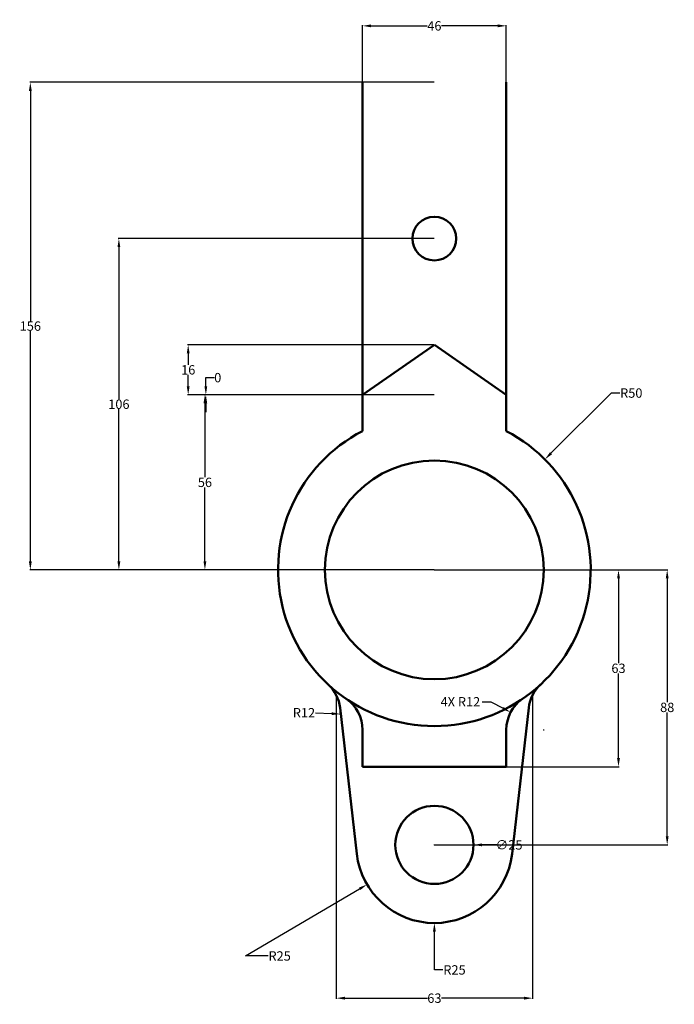
# Model space of a CAD drawing. Units: millimetres. Extents: x 164 to 765, y 152 to 486.
# Tile 1 of 2: x 164 to 373, y 158 to 473. Entities that reach past the tile are written whole.
import ezdxf

# ---------------------------------------------------------------- set-up
doc = ezdxf.new("R2010")
doc.units = ezdxf.units.MM
doc.header["$MEASUREMENT"] = 0
doc.layers.add('M-DIMS', color=2, linetype='Continuous', lineweight=25)
doc.layers.add('M-OUTL', color=7, linetype='Continuous', lineweight=50)
doc.styles.get("Standard").update_dxf_attribs({"font": 'arial.ttf'})
doc.dimstyles.get("Standard").update_dxf_attribs({"dimtxt": 3, "dimasz": 2.75, "dimexe": 0.18, "dimexo": 0.0625, "dimgap": 0.09, "dimtad": 0, "dimtih": 1, "dimtoh": 1, "dimdec": 0, "dimzin": 0, "dimdsep": 46, "dimtxsty": 'Standard', "dimcen": 0.09, "dimadec": 0, "dimazin": 0, "dimtfac": 1, "dimtdec": 0, "dimtofl": 0, "dimtmove": 0, "dimatfit": 3, "dimfxl": 1, "dimtolj": 1, "dimtzin": 0, "dimarcsym": 0})

# ---------------------------------------------------------------- blocks, each defined once
blk = doc.blocks.new('*D1')
at = {"layer": 'Defpoints', "color": 0, "transparency": 16777216}
for p in [(265.14, 256.55), (327.94, 256.55), (327.94, 159.6)]:
    blk.add_point(p, dxfattribs=at)
at = {"layer": 'M-DIMS', "color": 0, "lineweight": -2, "transparency": 16777216}
for p, q in [((265.14, 256.49), (265.14, 159.42)), ((327.94, 256.49), (327.94, 159.42)), ((267.89, 159.6), (294.29, 159.6)), ((325.19, 159.6), (298.79, 159.6))]:
    blk.add_line(p, q, dxfattribs=at)
at = {"layer": 'M-DIMS', "color": 0, "transparency": 16777216}
for points in [[(267.89, 160.06), (267.89, 159.14), (265.14, 159.6)], [(325.19, 160.06), (325.19, 159.14), (327.94, 159.6)]]:
    blk.add_solid(points, dxfattribs=at)
at = {"layer": 'M-DIMS', "color": 0, "transparency": 16777216, "insert": (296.54, 159.6), "char_height": 3, "attachment_point": 5}
blk.add_mtext('\\A1;63', dxfattribs=at)
blk = doc.blocks.new('*D2')
at = {"layer": 'Defpoints', "color": 0, "transparency": 16777216}
for p in [(296.54, 296.64), (371.02, 296.64), (296.54, 208.64)]:
    blk.add_point(p, dxfattribs=at)
at = {"layer": 'M-DIMS', "color": 0, "lineweight": -2, "transparency": 16777216}
for p, q in [((296.6, 296.64), (371.2, 296.64)), ((371.02, 293.89), (371.02, 254.26)), ((371.02, 211.39), (371.02, 251.02)), ((296.6, 208.64), (371.2, 208.64))]:
    blk.add_line(p, q, dxfattribs=at)
at = {"layer": 'M-DIMS', "color": 0, "transparency": 16777216}
for points in [[(370.56, 293.89), (371.48, 293.89), (371.02, 296.64)], [(370.56, 211.39), (371.48, 211.39), (371.02, 208.64)]]:
    blk.add_solid(points, dxfattribs=at)
at = {"layer": 'M-DIMS', "color": 0, "transparency": 16777216, "insert": (371.02, 252.64), "char_height": 3, "attachment_point": 5}
blk.add_mtext('\\A1;88', dxfattribs=at)
blk = doc.blocks.new('*D3')
at = {"layer": 'Defpoints', "color": 0, "transparency": 16777216}
for p in [(296.54, 296.64), (355.44, 296.64), (296.54, 233.64)]:
    blk.add_point(p, dxfattribs=at)
at = {"layer": 'M-DIMS', "color": 0, "lineweight": -2, "transparency": 16777216}
for p, q in [((296.6, 296.64), (355.62, 296.64)), ((355.44, 293.89), (355.44, 266.77)), ((355.44, 236.39), (355.44, 263.52)), ((296.6, 233.64), (355.62, 233.64))]:
    blk.add_line(p, q, dxfattribs=at)
at = {"layer": 'M-DIMS', "color": 0, "transparency": 16777216}
for points in [[(354.98, 293.89), (355.9, 293.89), (355.44, 296.64)], [(354.98, 236.39), (355.9, 236.39), (355.44, 233.64)]]:
    blk.add_solid(points, dxfattribs=at)
at = {"layer": 'M-DIMS', "color": 0, "transparency": 16777216, "insert": (355.44, 265.14), "char_height": 3, "attachment_point": 5}
blk.add_mtext('\\A1;63', dxfattribs=at)
blk = doc.blocks.new('*D4')
at = {"layer": 'Defpoints', "color": 0, "transparency": 16777216}
for p in [(273.54, 470.7), (273.54, 452.64), (319.54, 452.64)]:
    blk.add_point(p, dxfattribs=at)
at = {"layer": 'M-DIMS', "color": 0, "lineweight": -2, "transparency": 16777216}
for p, q in [((273.54, 452.71), (273.54, 470.88)), ((276.29, 470.7), (294.24, 470.7)), ((316.79, 470.7), (298.84, 470.7)), ((319.54, 452.71), (319.54, 470.88))]:
    blk.add_line(p, q, dxfattribs=at)
at = {"layer": 'M-DIMS', "color": 0, "transparency": 16777216}
for points in [[(276.29, 471.16), (276.29, 470.24), (273.54, 470.7)], [(316.79, 471.16), (316.79, 470.24), (319.54, 470.7)]]:
    blk.add_solid(points, dxfattribs=at)
at = {"layer": 'M-DIMS', "color": 0, "transparency": 16777216, "insert": (296.54, 470.7), "char_height": 3, "attachment_point": 5}
blk.add_mtext('\\A1;46', dxfattribs=at)
blk = doc.blocks.new('*D5')
at = {"layer": 'Defpoints', "color": 0, "transparency": 16777216}
for p in [(223.13, 352.64), (296.54, 352.64), (296.54, 296.64)]:
    blk.add_point(p, dxfattribs=at)
at = {"layer": 'M-DIMS', "color": 0, "lineweight": -2, "transparency": 16777216}
for p, q in [((296.48, 352.64), (222.95, 352.64)), ((223.13, 349.89), (223.13, 326.26)), ((223.13, 299.39), (223.13, 323.02)), ((296.48, 296.64), (222.95, 296.64))]:
    blk.add_line(p, q, dxfattribs=at)
at = {"layer": 'M-DIMS', "color": 0, "transparency": 16777216}
for points in [[(222.67, 349.89), (223.58, 349.89), (223.13, 352.64)], [(222.67, 299.39), (223.58, 299.39), (223.13, 296.64)]]:
    blk.add_solid(points, dxfattribs=at)
at = {"layer": 'M-DIMS', "color": 0, "transparency": 16777216, "insert": (223.13, 324.64), "char_height": 3, "attachment_point": 5}
blk.add_mtext('\\A1;56', dxfattribs=at)
blk = doc.blocks.new('*D6')
at = {"layer": 'Defpoints', "color": 0, "transparency": 16777216}
for p in [(223.42, 352.64), (273.54, 352.64), (273.54, 352.64)]:
    blk.add_point(p, dxfattribs=at)
at = {"layer": 'M-DIMS', "color": 0, "lineweight": -2, "transparency": 16777216}
for p, q in [((223.42, 355.39), (223.42, 358.14)), ((223.42, 358.14), (226.17, 358.14)), ((273.48, 352.64), (223.24, 352.64)), ((273.48, 352.64), (223.24, 352.64)), ((223.42, 349.89), (223.42, 347.14))]:
    blk.add_line(p, q, dxfattribs=at)
at = {"layer": 'M-DIMS', "color": 0, "transparency": 16777216}
for points in [[(222.96, 355.39), (223.87, 355.39), (223.42, 352.64)], [(222.96, 349.89), (223.87, 349.89), (223.42, 352.64)]]:
    blk.add_solid(points, dxfattribs=at)
at = {"layer": 'M-DIMS', "color": 0, "transparency": 16777216, "insert": (227.23, 358.14), "char_height": 3, "attachment_point": 5}
blk.add_mtext('\\A1;0', dxfattribs=at)
blk = doc.blocks.new('*D7')
at = {"layer": 'Defpoints', "color": 0, "transparency": 16777216}
for p in [(195.6, 402.64), (296.54, 402.64), (296.54, 296.64)]:
    blk.add_point(p, dxfattribs=at)
at = {"layer": 'M-DIMS', "color": 0, "lineweight": -2, "transparency": 16777216}
for p, q in [((296.48, 402.64), (195.42, 402.64)), ((195.6, 399.89), (195.6, 351.26)), ((195.6, 299.39), (195.6, 348.02)), ((296.48, 296.64), (195.42, 296.64))]:
    blk.add_line(p, q, dxfattribs=at)
at = {"layer": 'M-DIMS', "color": 0, "transparency": 16777216}
for points in [[(195.14, 399.89), (196.06, 399.89), (195.6, 402.64)], [(195.14, 299.39), (196.06, 299.39), (195.6, 296.64)]]:
    blk.add_solid(points, dxfattribs=at)
at = {"layer": 'M-DIMS', "color": 0, "transparency": 16777216, "insert": (195.6, 349.64), "char_height": 3, "attachment_point": 5}
blk.add_mtext('\\A1;106', dxfattribs=at)
blk = doc.blocks.new('*D8')
at = {"layer": 'Defpoints', "color": 0, "transparency": 16777216}
for p in [(167.27, 452.64), (296.54, 452.64), (296.54, 296.64)]:
    blk.add_point(p, dxfattribs=at)
at = {"layer": 'M-DIMS', "color": 0, "lineweight": -2, "transparency": 16777216}
for p, q in [((296.48, 452.64), (167.09, 452.64)), ((167.27, 449.89), (167.27, 376.26)), ((167.27, 299.39), (167.27, 373.02)), ((296.48, 296.64), (167.09, 296.64))]:
    blk.add_line(p, q, dxfattribs=at)
at = {"layer": 'M-DIMS', "color": 0, "transparency": 16777216}
for points in [[(166.81, 449.89), (167.73, 449.89), (167.27, 452.64)], [(166.81, 299.39), (167.73, 299.39), (167.27, 296.64)]]:
    blk.add_solid(points, dxfattribs=at)
at = {"layer": 'M-DIMS', "color": 0, "transparency": 16777216, "insert": (167.27, 374.64), "char_height": 3, "attachment_point": 5}
blk.add_mtext('\\A1;156', dxfattribs=at)
blk = doc.blocks.new('*D9')
at = {"layer": 'Defpoints', "color": 0, "transparency": 16777216}
for p in [(296.54, 208.64), (274.99, 195.97)]:
    blk.add_point(p, dxfattribs=at)
at = {"layer": 'M-DIMS', "color": 0, "lineweight": -2, "transparency": 16777216}
for p, q in [((296.45, 208.64), (296.63, 208.64)), ((296.54, 208.55), (296.54, 208.73)), ((236.08, 173.1), (272.62, 194.58)), ((243.34, 173.1), (236.08, 173.1))]:
    blk.add_line(p, q, dxfattribs=at)
at = {"layer": 'M-DIMS', "color": 0, "transparency": 16777216}
blk.add_solid([(272.39, 194.97), (272.85, 194.18), (274.99, 195.97)], dxfattribs=at)
at = {"layer": 'M-DIMS', "color": 0, "transparency": 16777216, "insert": (247.03, 173.1), "char_height": 3, "attachment_point": 5}
blk.add_mtext('\\A1;R25', dxfattribs=at)
blk = doc.blocks.new('*D10')
at = {"layer": 'Defpoints', "color": 0, "transparency": 16777216}
for p in [(254.44, 251.13), (266.42, 250.49)]:
    blk.add_point(p, dxfattribs=at)
at = {"layer": 'M-DIMS', "color": 0, "lineweight": -2, "transparency": 16777216}
blk.add_line((258.47, 250.92), (263.68, 250.64), dxfattribs=at)
blk.add_arc((254.44, 251.13), 12, 356.11, 6.2266, dxfattribs=at)
at = {"layer": 'M-DIMS', "color": 0, "transparency": 16777216}
blk.add_solid([(263.7, 251.1), (263.65, 250.18), (266.42, 250.49)], dxfattribs=at)
at = {"layer": 'M-DIMS', "color": 0, "transparency": 16777216, "insert": (254.81, 250.92), "char_height": 3, "attachment_point": 5}
blk.add_mtext('\\A1;R12', dxfattribs=at)
blk = doc.blocks.new('*D27')
at = {"layer": 'Defpoints', "color": 0, "transparency": 16777216}
for p in [(217.78, 368.64), (296.54, 368.64), (273.54, 352.64)]:
    blk.add_point(p, dxfattribs=at)
at = {"layer": 'M-DIMS', "color": 0, "lineweight": -2, "transparency": 16777216}
for p, q in [((296.48, 368.64), (217.6, 368.64)), ((217.78, 365.89), (217.78, 362.26)), ((217.78, 355.39), (217.78, 359.02)), ((273.48, 352.64), (217.6, 352.64))]:
    blk.add_line(p, q, dxfattribs=at)
at = {"layer": 'M-DIMS', "color": 0, "transparency": 16777216}
for points in [[(217.32, 365.89), (218.23, 365.89), (217.78, 368.64)], [(217.32, 355.39), (218.23, 355.39), (217.78, 352.64)]]:
    blk.add_solid(points, dxfattribs=at)
at = {"layer": 'M-DIMS', "color": 0, "transparency": 16777216, "insert": (217.78, 360.64), "char_height": 3, "attachment_point": 5}
blk.add_mtext('\\A1;16', dxfattribs=at)
blk = doc.blocks.new('*D37')
at = {"layer": 'Defpoints', "color": 0, "transparency": 16777216}
for p in [(331.9, 332), (296.54, 296.64)]:
    blk.add_point(p, dxfattribs=at)
at = {"layer": 'M-DIMS', "color": 0, "lineweight": -2, "transparency": 16777216}
for p, q in [((353.11, 353.21), (333.84, 333.94)), ((355.86, 353.21), (353.11, 353.21)), ((296.45, 296.64), (296.63, 296.64)), ((296.54, 296.55), (296.54, 296.73))]:
    blk.add_line(p, q, dxfattribs=at)
at = {"layer": 'M-DIMS', "color": 0, "transparency": 16777216}
blk.add_solid([(333.52, 334.26), (334.17, 333.62), (331.9, 332)], dxfattribs=at)
at = {"layer": 'M-DIMS', "color": 0, "transparency": 16777216, "insert": (359.53, 353.21), "char_height": 3, "attachment_point": 5}
blk.add_mtext('\\A1;R50', dxfattribs=at)
blk = doc.blocks.new('*D38')
at = {"layer": 'Defpoints', "color": 0, "transparency": 16777216}
for p in [(284.04, 208.64), (309.04, 208.64)]:
    blk.add_point(p, dxfattribs=at)
at = {"layer": 'M-DIMS', "color": 0, "lineweight": -2, "transparency": 16777216}
for p, q in [((296.45, 208.64), (296.63, 208.64)), ((296.54, 208.55), (296.54, 208.73)), ((316.54, 208.64), (311.79, 208.64))]:
    blk.add_line(p, q, dxfattribs=at)
at = {"layer": 'M-DIMS', "color": 0, "transparency": 16777216}
blk.add_solid([(311.79, 209.1), (311.79, 208.18), (309.04, 208.64)], dxfattribs=at)
at = {"layer": 'M-DIMS', "color": 0, "transparency": 16777216, "insert": (320.42, 208.64), "char_height": 3, "attachment_point": 5}
blk.add_mtext('\\A1;∅25', dxfattribs=at)
blk = doc.blocks.new('*D39')
at = {"layer": 'Defpoints', "color": 0, "transparency": 16777216}
for p in [(296.54, 208.64), (296.54, 183.64)]:
    blk.add_point(p, dxfattribs=at)
at = {"layer": 'M-DIMS', "color": 0, "lineweight": -2, "transparency": 16777216}
for p, q in [((296.45, 208.64), (296.63, 208.64)), ((296.54, 208.55), (296.54, 208.73)), ((296.54, 168.64), (296.54, 180.89)), ((299.29, 168.64), (296.54, 168.64))]:
    blk.add_line(p, q, dxfattribs=at)
at = {"layer": 'M-DIMS', "color": 0, "transparency": 16777216}
blk.add_solid([(297, 180.89), (296.08, 180.89), (296.54, 183.64)], dxfattribs=at)
at = {"layer": 'M-DIMS', "color": 0, "transparency": 16777216, "insert": (302.97, 168.64), "char_height": 3, "attachment_point": 5}
blk.add_mtext('\\A1;R25', dxfattribs=at)
blk = doc.blocks.new('*D40')
at = {"layer": 'Defpoints', "color": 0, "transparency": 16777216}
for p in [(320.93, 251.07), (331.54, 245.47)]:
    blk.add_point(p, dxfattribs=at)
at = {"layer": 'M-DIMS', "color": 0, "lineweight": -2, "transparency": 16777216}
for p, q in [((311.81, 254.43), (314.56, 254.43)), ((314.56, 254.43), (318.49, 252.35)), ((331.45, 245.47), (331.63, 245.47)), ((331.54, 245.38), (331.54, 245.56))]:
    blk.add_line(p, q, dxfattribs=at)
at = {"layer": 'M-DIMS', "color": 0, "transparency": 16777216}
blk.add_solid([(318.71, 252.75), (318.28, 251.94), (320.93, 251.07)], dxfattribs=at)
at = {"layer": 'M-DIMS', "color": 0, "transparency": 16777216, "insert": (304.86, 254.43), "char_height": 3, "attachment_point": 5}
blk.add_mtext('\\A1;4X R12', dxfattribs=at)

msp = doc.modelspace()

# ---------------------------------------------------------------- linework, layer by layer
at = {"layer": 'M-OUTL'}
for p, q in [((273.5388, 341.039), (273.5388, 452.6431)), ((319.5388, 341.039), (319.5388, 452.6431)), ((273.5388, 352.6431), (296.5388, 368.6431)), ((296.5388, 368.6431), (319.5388, 352.6431)), ((271.7008, 205.8022), (266.3605, 252.4926)), ((321.3769, 205.8022), (326.7172, 252.4926)), ((273.5388, 245.4669), (273.5388, 233.6431)), ((319.5388, 245.4669), (319.5388, 233.6431)), ((273.5388, 233.6431), (319.5388, 233.6431))]:
    msp.add_line(p, q, dxfattribs=at)
for centre, radius in [((296.5388, 402.6431), 7), ((296.5388, 296.6431), 35), ((296.5388, 208.6431), 12.5)]:
    msp.add_circle(centre, radius, dxfattribs=at)
for centre, radius, start, end in [((296.5388, 296.6431), 50, 117.387108, 62.612892), ((254.4382, 251.1289), 12, 6.524979, 47.231113), ((338.6395, 251.1289), 12, 132.768887, 173.475021), ((261.5388, 245.4669), 12, 0, 55.631303), ((331.5388, 245.4669), 12, 124.368697, 180), ((296.5388, 208.6431), 25, 186.524979, 353.475021)]:
    msp.add_arc(centre, radius, start, end, dxfattribs=at)

# ---------------------------------------------------------------- dimensions: what is measured, and where the dimension line sits
at = {"layer": 'M-DIMS'}
for base, p1, p2, angle, override, picture, middle in [((273.5388, 470.7032), (319.5388, 452.6431), (273.5388, 452.6431), 180, {"dimclrd": 0, "dimclre": 0, "dimclrt": 0}, '*D4', (296.5388, 470.7032)), ((167.2722, 452.6431), (296.5388, 296.6431), (296.5388, 452.6431), 90, {"dimclrd": 0, "dimclre": 0, "dimclrt": 0}, '*D8', (167.2722, 374.6431)), ((195.6026, 402.6431), (296.5388, 296.6431), (296.5388, 402.6431), 90, {"dimclrd": 0, "dimclre": 0, "dimclrt": 0}, '*D7', (195.6026, 349.6431)), ((217.7755, 368.6431), (273.5388, 352.6431), (296.5388, 368.6431), 90, {"dimdec": 0, "dimlfac": 1, "dimrnd": 0, "dimzin": 0, "dimdsep": 46, "dimlunit": 2}, '*D27', (217.7755, 360.6431)), ((223.4151262394, 352.6430700485), (273.5388456179, 352.6430700485), (273.5388456179, 352.6430700485), 90, {"dimclrd": 0, "dimclre": 0, "dimclrt": 0}, '*D6', (227.2332981357, 358.1430700485)), ((223.1255, 352.6431), (296.5388, 296.6431), (296.5388, 352.6431), 90, {"dimclrd": 0, "dimclre": 0, "dimclrt": 0}, '*D5', (223.1255, 324.6431)), ((371.0219, 296.6431), (296.5388, 208.6431), (296.5388, 296.6431), 90, {"dimclrd": 0, "dimclre": 0, "dimclrt": 0}, '*D2', (371.0219, 252.6431)), ((355.4423, 296.6431), (296.5388, 233.6431), (296.5388, 296.6431), 90, {"dimclrd": 0, "dimclre": 0, "dimclrt": 0}, '*D3', (355.4423, 265.1431)), ((327.9358, 159.6015), (265.1418, 256.5541), (327.9358, 256.5541), 180, {"dimclrd": 0, "dimclre": 0, "dimclrt": 0}, '*D1', (296.5388, 159.6015))]:
    dim = msp.add_linear_dim(base=base, p1=p1, p2=p2, angle=angle, dimstyle='Standard', override=override, dxfattribs=at)
    dim.commit()
    dim.dimension.update_dxf_attribs({"geometry": picture, "text_midpoint": middle})
for center, mpoint, override, picture, middle in [((296.5388, 296.6431), (331.8963, 331.9963), {"dimdec": 0, "dimlfac": 1, "dimrnd": 0, "dimzin": 0, "dimdsep": 46, "dimlunit": 2}, '*D37', (359.5299, 353.2082)), ((254.4382, 251.1289), (266.4214, 250.4945), {"dimclrd": 0, "dimclre": 0, "dimclrt": 0}, '*D10', (258.4693, 250.9155)), ((296.5388, 208.6431), (274.9879, 195.9719), {"dimclrd": 0, "dimclre": 0, "dimclrt": 0}, '*D9', (247.0289, 173.0974)), ((296.5388, 208.6431), (296.539, 183.6431), {"dimdec": 0, "dimlfac": 1, "dimrnd": 0, "dimzin": 0, "dimdsep": 46, "dimlunit": 2}, '*D39', (302.9746, 168.6431))]:
    dim = msp.add_radius_dim(center=center, mpoint=mpoint, dimstyle='Standard', override=override, dxfattribs=at)
    dim.commit()
    dim.dimension.update_dxf_attribs({"geometry": picture, "text_midpoint": middle, "dimtype": 164})
dim = msp.add_radius_dim(center=(331.5388, 245.4669), mpoint=(320.9251, 251.0659), text='4X <>', dimstyle='Standard', override={"dimdec": 0, "dimlfac": 1, "dimrnd": 0, "dimzin": 0, "dimdsep": 46, "dimlunit": 2}, dxfattribs=at)
dim.commit()
dim.dimension.update_dxf_attribs({"geometry": '*D40', "text_midpoint": (304.8646, 254.4253), "dimtype": 164})
dim = msp.add_diameter_dim_2p(p1=(284.0388, 208.6431), p2=(309.0388, 208.643), dimstyle='Standard', override={"dimdec": 0, "dimlfac": 1, "dimrnd": 0, "dimzin": 0, "dimdsep": 46, "dimlunit": 2}, dxfattribs=at)
dim.commit()
dim.dimension.update_dxf_attribs({"geometry": '*D38', "text_midpoint": (316.5388, 208.643), "dimtype": 163})

doc.saveas('drawing.dxf')
